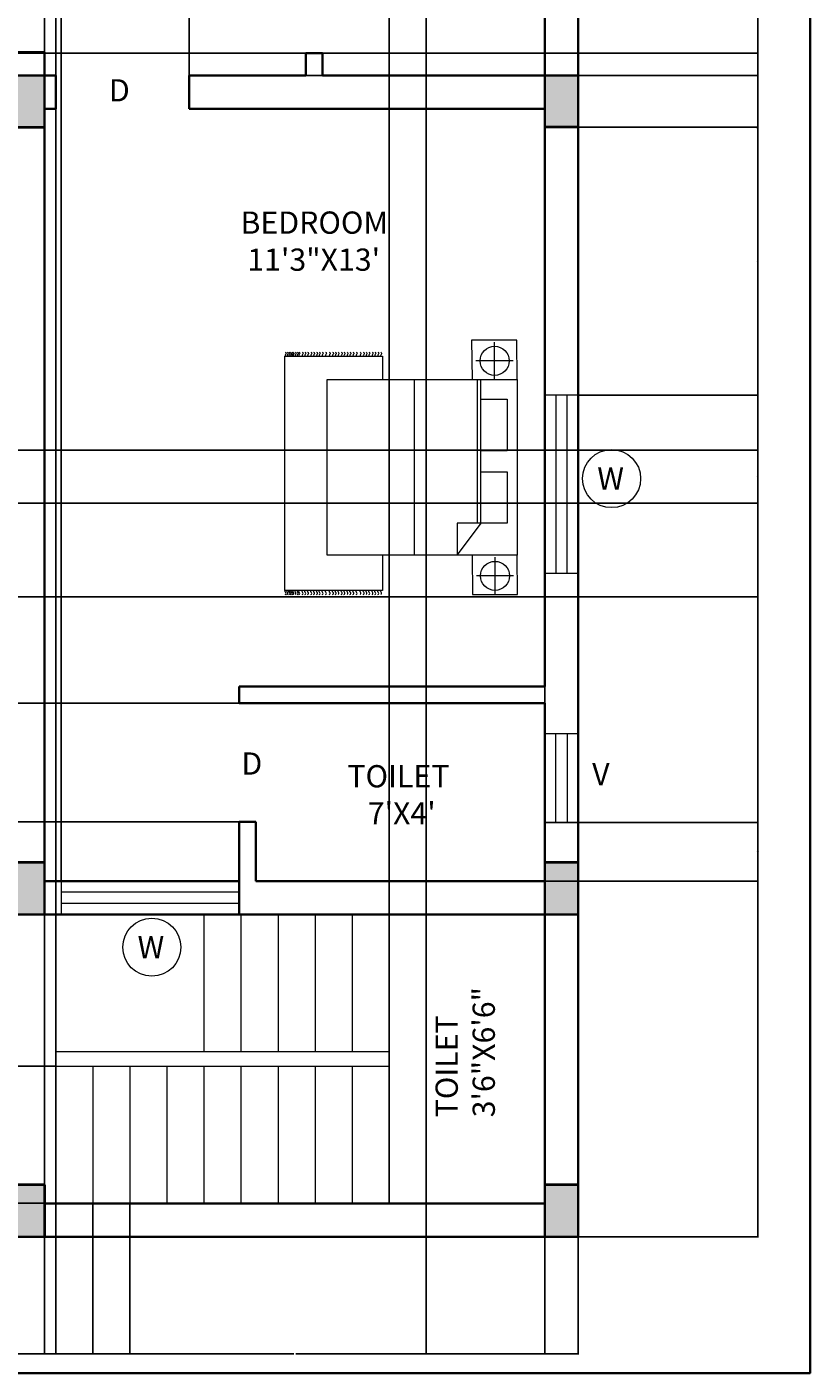
# Model space of a CAD drawing. Units: inches. Extents: x 2243 to 2668, y 14541 to 15226.
# Tile 2 of 5: x 2456 to 2668, y 14541 to 14904. Entities that reach past the tile are written whole.
import ezdxf

# ---------------------------------------------------------------- set-up
doc = ezdxf.new("R2010")
doc.units = ezdxf.units.IN
doc.header["$MEASUREMENT"] = 0
for name, color, linetype, lineweight in [('A-ANNO-DIMS', 2, 'Continuous', 18), ('A-ANNO-SYMB', 3, 'Continuous', 18), ('A-ANNO-TTLB', 7, 'Continuous', 35), ('A-AREA-IDEN', 7, 'Continuous', 18), ('A-COLS', 7, 'Continuous', 40), ('A-COLS-PATT', 7, 'Continuous', 13), ('A-FLOR-STRS', 7, 'Continuous', 18), ('A-FURN', 8, 'Continuous', 18), ('A-GLAZ', 4, 'Continuous', 18), ('A-GLAZ-VENT', 4, 'Continuous', 18), ('A-WALL', 7, 'Continuous', 35)]:
    doc.layers.add(name, color=color, linetype=linetype, lineweight=lineweight)
doc.styles.get("Standard").update_dxf_attribs({"font": 'arial.ttf'})
doc.dimstyles.get("Standard").update_dxf_attribs({"dimtxt": 0.18, "dimasz": 0.18, "dimexe": 0.18, "dimexo": 0.0625, "dimgap": 0.09, "dimtad": 0, "dimtih": 1, "dimtoh": 1, "dimdec": 4, "dimzin": 0, "dimdsep": 46, "dimtxsty": 'Standard', "dimcen": 0.09, "dimadec": 0, "dimazin": 0, "dimtfac": 1, "dimtdec": 4, "dimtofl": 0, "dimtmove": 0, "dimatfit": 3, "dimfxl": 1, "dimtolj": 1, "dimtzin": 0, "dimarcsym": 0})

# ---------------------------------------------------------------- blocks, each defined once
blk = doc.blocks.new('BED-DOUBLE-WITH-NIGHTSTANDS')
for p, q in [((56.59, 58.08), (56.59, 68.14)), ((0, 64.36), (26.37, 64.36)), ((0, 1.12), (0, 64.36)), ((26.37, 64.36), (26.37, 58.06)), ((61.62, 63.11), (51.56, 63.11)), ((34.96, 10.66), (34.96, 58.08)), ((52, 19.27), (52, 58.08)), ((52.82, 19.32), (52.82, 58.08)), ((52.82, 19.32), (46.47, 10.71)), ((52.82, 19.27), (46.47, 19.27)), ((46.47, 19.27), (46.47, 10.71)), ((26.37, 10.66), (26.37, 1.12)), ((56.69, 0.03), (56.69, 10.09)), ((61.72, 5.06), (51.66, 5.06)), ((26.37, 1.12), (0, 1.12))]:
    blk.add_line(p, q)
for points in [[(50.39, 68.71), (50.5, 58.08), (62.68, 58.08), (62.58, 68.71)], [(62.68, 10.66), (11.36, 10.66), (11.36, 58.08), (62.68, 58.08)], [(59.98, 38.83), (52.82, 38.83), (52.82, 52.73), (59.98, 52.73)], [(59.98, 19.27), (52.82, 19.27), (52.82, 33.16), (59.98, 33.16)], [(50.5, 10.66), (50.6, 0.03), (62.78, 0.03), (62.68, 10.66)]]:
    blk.add_lwpolyline(points, close=True)
for centre in [(56.59, 63.11), (56.69, 5.06)]:
    blk.add_circle(centre, 3.92)
for points, knots in [([(0.07, 65.48), (0.19, 65.39), (0.43, 65.19), (0.19, 64.85), (0.02, 64.57), (0.13, 64.42), (0.18, 64.36)], [0, 0, 0, 0, 0.400747, 0.791423, 1.067667, 1.29709, 1.29709, 1.29709, 1.29709]), ([(0.57, 65.48), (0.7, 65.39), (0.94, 65.19), (0.7, 64.85), (0.52, 64.57), (0.63, 64.42), (0.68, 64.36)], [0, 0, 0, 0, 0.400747, 0.791423, 1.067667, 1.29709, 1.29709, 1.29709, 1.29709]), ([(1.06, 65.48), (1.18, 65.39), (1.42, 65.19), (1.18, 64.85), (1.01, 64.57), (1.11, 64.42), (1.16, 64.36)], [0, 0, 0, 0, 0.400747, 0.791423, 1.067667, 1.29709, 1.29709, 1.29709, 1.29709]), ([(1.46, 65.48), (1.58, 65.39), (1.82, 65.19), (1.58, 64.85), (1.4, 64.57), (1.51, 64.42), (1.56, 64.36)], [0, 0, 0, 0, 0.400747, 0.791423, 1.067667, 1.29709, 1.29709, 1.29709, 1.29709]), ([(1.88, 65.48), (2, 65.39), (2.24, 65.19), (2, 64.85), (1.82, 64.57), (1.93, 64.42), (1.98, 64.36)], [0, 0, 0, 0, 0.400747, 0.791423, 1.067667, 1.29709, 1.29709, 1.29709, 1.29709]), ([(2.18, 65.48), (2.31, 65.39), (2.55, 65.19), (2.31, 64.85), (2.13, 64.57), (2.24, 64.42), (2.29, 64.36)], [0, 0, 0, 0, 0.400747, 0.791423, 1.067667, 1.29709, 1.29709, 1.29709, 1.29709]), ([(2.76, 65.48), (2.88, 65.39), (3.12, 65.19), (2.88, 64.85), (2.71, 64.57), (2.81, 64.42), (2.86, 64.36)], [0, 0, 0, 0, 0.400747, 0.791423, 1.067667, 1.29709, 1.29709, 1.29709, 1.29709]), ([(3.32, 65.48), (3.45, 65.39), (3.7, 65.2), (3.44, 64.85), (3.27, 64.57), (3.38, 64.42), (3.43, 64.36)], [0, 0, 0, 0, 0.407265, 0.802015, 1.07826, 1.307683, 1.307683, 1.307683, 1.307683]), ([(3.75, 65.48), (3.88, 65.39), (4.11, 65.19), (3.88, 64.85), (3.7, 64.57), (3.81, 64.42), (3.86, 64.36)], [0, 0, 0, 0, 0.400747, 0.791423, 1.067667, 1.29709, 1.29709, 1.29709, 1.29709]), ([(4.64, 65.48), (4.76, 65.39), (5, 65.19), (4.76, 64.85), (4.58, 64.57), (4.69, 64.42), (4.74, 64.36)], [0, 0, 0, 0, 0.400747, 0.791423, 1.067667, 1.29709, 1.29709, 1.29709, 1.29709]), ([(5.36, 65.48), (5.49, 65.39), (5.73, 65.19), (5.49, 64.85), (5.31, 64.57), (5.42, 64.42), (5.47, 64.36)], [0, 0, 0, 0, 0.400747, 0.791423, 1.067667, 1.29709, 1.29709, 1.29709, 1.29709]), ([(6.12, 65.48), (6.24, 65.39), (6.48, 65.19), (6.24, 64.85), (6.07, 64.57), (6.17, 64.42), (6.22, 64.36)], [0, 0, 0, 0, 0.400747, 0.791423, 1.067667, 1.29709, 1.29709, 1.29709, 1.29709]), ([(7, 65.48), (7.12, 65.39), (7.36, 65.19), (7.12, 64.85), (6.95, 64.57), (7.05, 64.42), (7.1, 64.36)], [0, 0, 0, 0, 0.400747, 0.791423, 1.067667, 1.29709, 1.29709, 1.29709, 1.29709]), ([(7.73, 65.48), (7.85, 65.39), (8.09, 65.19), (7.85, 64.85), (7.68, 64.57), (7.78, 64.42), (7.83, 64.36)], [0, 0, 0, 0, 0.400747, 0.791423, 1.067667, 1.29709, 1.29709, 1.29709, 1.29709]), ([(8.54, 65.48), (8.66, 65.39), (8.9, 65.19), (8.66, 64.85), (8.49, 64.57), (8.6, 64.42), (8.65, 64.36)], [0, 0, 0, 0, 0.400747, 0.791423, 1.067667, 1.29709, 1.29709, 1.29709, 1.29709]), ([(9.23, 65.48), (9.35, 65.39), (9.59, 65.19), (9.35, 64.85), (9.18, 64.57), (9.29, 64.42), (9.34, 64.36)], [0, 0, 0, 0, 0.400747, 0.791423, 1.067667, 1.29709, 1.29709, 1.29709, 1.29709]), ([(10.05, 65.48), (10.17, 65.39), (10.41, 65.19), (10.17, 64.85), (10, 64.57), (10.1, 64.42), (10.15, 64.36)], [0, 0, 0, 0, 0.400747, 0.791423, 1.067667, 1.29709, 1.29709, 1.29709, 1.29709]), ([(10.93, 65.48), (11.05, 65.39), (11.29, 65.19), (11.05, 64.85), (10.88, 64.57), (10.99, 64.42), (11.03, 64.36)], [0, 0, 0, 0, 0.400747, 0.791423, 1.067667, 1.29709, 1.29709, 1.29709, 1.29709]), ([(11.97, 65.48), (12.09, 65.39), (12.33, 65.19), (12.09, 64.85), (11.92, 64.57), (12.02, 64.42), (12.07, 64.36)], [0, 0, 0, 0, 0.400747, 0.791423, 1.067667, 1.29709, 1.29709, 1.29709, 1.29709]), ([(12.85, 65.48), (12.97, 65.39), (13.21, 65.19), (12.97, 64.85), (12.8, 64.57), (12.9, 64.42), (12.95, 64.36)], [0, 0, 0, 0, 0.400747, 0.791423, 1.067667, 1.29709, 1.29709, 1.29709, 1.29709]), ([(13.58, 65.48), (13.7, 65.39), (13.94, 65.19), (13.7, 64.85), (13.53, 64.57), (13.63, 64.42), (13.68, 64.36)], [0, 0, 0, 0, 0.400747, 0.791423, 1.067667, 1.29709, 1.29709, 1.29709, 1.29709]), ([(14.33, 65.48), (14.45, 65.39), (14.69, 65.19), (14.45, 64.85), (14.28, 64.57), (14.38, 64.42), (14.43, 64.36)], [0, 0, 0, 0, 0.400747, 0.791423, 1.067667, 1.29709, 1.29709, 1.29709, 1.29709]), ([(15.21, 65.48), (15.33, 65.39), (15.57, 65.19), (15.33, 64.85), (15.16, 64.57), (15.27, 64.42), (15.32, 64.36)], [0, 0, 0, 0, 0.400747, 0.791423, 1.067667, 1.29709, 1.29709, 1.29709, 1.29709]), ([(15.94, 65.48), (16.06, 65.39), (16.3, 65.19), (16.06, 64.85), (15.89, 64.57), (15.99, 64.42), (16.04, 64.36)], [0, 0, 0, 0, 0.400747, 0.791423, 1.067667, 1.29709, 1.29709, 1.29709, 1.29709]), ([(16.76, 65.48), (16.88, 65.39), (17.12, 65.19), (16.88, 64.85), (16.7, 64.57), (16.81, 64.42), (16.86, 64.36)], [0, 0, 0, 0, 0.400747, 0.791423, 1.067667, 1.29709, 1.29709, 1.29709, 1.29709]), ([(17.53, 65.48), (17.65, 65.39), (17.89, 65.19), (17.65, 64.85), (17.48, 64.57), (17.59, 64.42), (17.64, 64.36)], [0, 0, 0, 0, 0.400747, 0.791423, 1.067667, 1.29709, 1.29709, 1.29709, 1.29709]), ([(18.35, 65.48), (18.47, 65.39), (18.71, 65.19), (18.47, 64.85), (18.3, 64.57), (18.4, 64.42), (18.45, 64.36)], [0, 0, 0, 0, 0.400747, 0.791423, 1.067667, 1.29709, 1.29709, 1.29709, 1.29709]), ([(19.23, 65.48), (19.35, 65.39), (19.59, 65.19), (19.35, 64.85), (19.18, 64.57), (19.29, 64.42), (19.33, 64.36)], [0, 0, 0, 0, 0.400747, 0.791423, 1.067667, 1.29709, 1.29709, 1.29709, 1.29709]), ([(20.27, 65.48), (20.39, 65.39), (20.63, 65.19), (20.39, 64.85), (20.22, 64.57), (20.32, 64.42), (20.37, 64.36)], [0, 0, 0, 0, 0.400747, 0.791423, 1.067667, 1.29709, 1.29709, 1.29709, 1.29709]), ([(21.15, 65.48), (21.27, 65.39), (21.51, 65.19), (21.27, 64.85), (21.1, 64.57), (21.21, 64.42), (21.25, 64.36)], [0, 0, 0, 0, 0.400747, 0.791423, 1.067667, 1.29709, 1.29709, 1.29709, 1.29709]), ([(21.88, 65.48), (22, 65.39), (22.24, 65.19), (22, 64.85), (21.83, 64.57), (21.93, 64.42), (21.98, 64.36)], [0, 0, 0, 0, 0.400747, 0.791423, 1.067667, 1.29709, 1.29709, 1.29709, 1.29709]), ([(22.63, 65.48), (22.75, 65.39), (22.99, 65.19), (22.75, 64.85), (22.58, 64.57), (22.69, 64.42), (22.73, 64.36)], [0, 0, 0, 0, 0.400747, 0.791423, 1.067667, 1.29709, 1.29709, 1.29709, 1.29709]), ([(23.51, 65.48), (23.63, 65.39), (23.87, 65.19), (23.63, 64.85), (23.46, 64.57), (23.57, 64.42), (23.62, 64.36)], [0, 0, 0, 0, 0.400747, 0.791423, 1.067667, 1.29709, 1.29709, 1.29709, 1.29709]), ([(24.24, 65.48), (24.36, 65.39), (24.6, 65.19), (24.36, 64.85), (24.19, 64.57), (24.3, 64.42), (24.34, 64.36)], [0, 0, 0, 0, 0.400747, 0.791423, 1.067667, 1.29709, 1.29709, 1.29709, 1.29709]), ([(25.06, 65.48), (25.18, 65.39), (25.42, 65.19), (25.18, 64.85), (25.01, 64.57), (25.11, 64.42), (25.16, 64.36)], [0, 0, 0, 0, 0.400747, 0.791423, 1.067667, 1.29709, 1.29709, 1.29709, 1.29709]), ([(25.84, 65.48), (25.96, 65.39), (26.2, 65.19), (25.96, 64.85), (25.78, 64.57), (25.89, 64.42), (25.94, 64.36)], [0, 0, 0, 0, 0.400747, 0.791423, 1.067667, 1.29709, 1.29709, 1.29709, 1.29709]), ([(0.07, 0), (0.19, 0.1), (0.43, 0.29), (0.19, 0.63), (0.02, 0.91), (0.13, 1.06), (0.18, 1.13)], [0, 0, 0, 0, 0.400747, 0.791423, 1.067667, 1.29709, 1.29709, 1.29709, 1.29709]), ([(0.55, 0), (0.67, 0.1), (0.91, 0.29), (0.67, 0.63), (0.49, 0.91), (0.6, 1.06), (0.65, 1.13)], [0, 0, 0, 0, 0.400747, 0.791423, 1.067667, 1.29709, 1.29709, 1.29709, 1.29709]), ([(1.03, 0), (1.15, 0.1), (1.39, 0.29), (1.15, 0.63), (0.98, 0.91), (1.09, 1.06), (1.13, 1.13)], [0, 0, 0, 0, 0.400747, 0.791423, 1.067667, 1.29709, 1.29709, 1.29709, 1.29709]), ([(1.43, 0), (1.55, 0.1), (1.79, 0.29), (1.55, 0.63), (1.38, 0.91), (1.48, 1.06), (1.53, 1.13)], [0, 0, 0, 0, 0.400747, 0.791423, 1.067667, 1.29709, 1.29709, 1.29709, 1.29709]), ([(1.85, 0), (1.97, 0.1), (2.21, 0.29), (1.97, 0.63), (1.8, 0.91), (1.9, 1.05), (1.94, 1.12)], [0, 0, 0, 0, 0.400747, 0.791423, 1.067667, 1.283686, 1.283686, 1.283686, 1.283686]), ([(2.16, 0), (2.28, 0.1), (2.52, 0.29), (2.28, 0.63), (2.11, 0.91), (2.21, 1.05), (2.25, 1.12)], [0, 0, 0, 0, 0.400747, 0.791423, 1.067667, 1.283686, 1.283686, 1.283686, 1.283686]), ([(2.73, 0), (2.85, 0.1), (3.09, 0.29), (2.85, 0.63), (2.68, 0.91), (2.78, 1.05), (2.82, 1.12)], [0, 0, 0, 0, 0.400747, 0.791423, 1.067667, 1.283686, 1.283686, 1.283686, 1.283686]), ([(3.32, 0), (3.45, 0.1), (3.69, 0.29), (3.45, 0.63), (3.27, 0.91), (3.38, 1.05), (3.42, 1.12)], [0, 0, 0, 0, 0.402903, 0.794912, 1.071156, 1.287177, 1.287177, 1.287177, 1.287177]), ([(3.75, 0), (3.88, 0.1), (4.11, 0.29), (3.88, 0.63), (3.7, 0.91), (3.8, 1.05), (3.85, 1.12)], [0, 0, 0, 0, 0.400747, 0.791423, 1.067667, 1.283686, 1.283686, 1.283686, 1.283686]), ([(4.64, 0), (4.76, 0.1), (5, 0.29), (4.76, 0.63), (4.59, 0.91), (4.69, 1.05), (4.73, 1.12)], [0, 0, 0, 0, 0.400747, 0.791423, 1.067667, 1.283686, 1.283686, 1.283686, 1.283686]), ([(5.36, 0), (5.49, 0.1), (5.73, 0.29), (5.49, 0.63), (5.31, 0.91), (5.42, 1.06), (5.47, 1.13)], [0, 0, 0, 0, 0.400747, 0.791423, 1.067667, 1.29709, 1.29709, 1.29709, 1.29709]), ([(6.12, 0), (6.24, 0.1), (6.48, 0.29), (6.24, 0.63), (6.07, 0.91), (6.17, 1.06), (6.22, 1.13)], [0, 0, 0, 0, 0.400747, 0.791423, 1.067667, 1.29709, 1.29709, 1.29709, 1.29709]), ([(7, 0), (7.12, 0.1), (7.36, 0.29), (7.12, 0.63), (6.95, 0.91), (7.05, 1.06), (7.1, 1.13)], [0, 0, 0, 0, 0.400747, 0.791423, 1.067667, 1.29709, 1.29709, 1.29709, 1.29709]), ([(7.73, 0), (7.85, 0.1), (8.09, 0.29), (7.85, 0.63), (7.68, 0.91), (7.78, 1.06), (7.83, 1.13)], [0, 0, 0, 0, 0.400747, 0.791423, 1.067667, 1.29709, 1.29709, 1.29709, 1.29709]), ([(8.54, 0), (8.66, 0.1), (8.9, 0.29), (8.66, 0.63), (8.49, 0.91), (8.6, 1.06), (8.65, 1.13)], [0, 0, 0, 0, 0.400747, 0.791423, 1.067667, 1.29709, 1.29709, 1.29709, 1.29709]), ([(9.23, 0), (9.35, 0.1), (9.59, 0.29), (9.35, 0.63), (9.18, 0.91), (9.29, 1.06), (9.34, 1.13)], [0, 0, 0, 0, 0.400747, 0.791423, 1.067667, 1.29709, 1.29709, 1.29709, 1.29709]), ([(10.05, 0), (10.17, 0.1), (10.41, 0.29), (10.17, 0.63), (10, 0.91), (10.1, 1.06), (10.15, 1.13)], [0, 0, 0, 0, 0.400747, 0.791423, 1.067667, 1.29709, 1.29709, 1.29709, 1.29709]), ([(10.93, 0), (11.05, 0.1), (11.29, 0.29), (11.05, 0.63), (10.88, 0.91), (10.99, 1.06), (11.03, 1.13)], [0, 0, 0, 0, 0.400747, 0.791423, 1.067667, 1.29709, 1.29709, 1.29709, 1.29709]), ([(11.97, 0), (12.09, 0.1), (12.33, 0.29), (12.09, 0.63), (11.92, 0.91), (12.02, 1.06), (12.07, 1.13)], [0, 0, 0, 0, 0.400747, 0.791423, 1.067667, 1.29709, 1.29709, 1.29709, 1.29709]), ([(12.85, 0), (12.97, 0.1), (13.21, 0.29), (12.97, 0.63), (12.8, 0.91), (12.9, 1.06), (12.95, 1.13)], [0, 0, 0, 0, 0.400747, 0.791423, 1.067667, 1.29709, 1.29709, 1.29709, 1.29709]), ([(13.58, 0), (13.7, 0.1), (13.94, 0.29), (13.7, 0.63), (13.53, 0.91), (13.63, 1.06), (13.68, 1.13)], [0, 0, 0, 0, 0.400747, 0.791423, 1.067667, 1.29709, 1.29709, 1.29709, 1.29709]), ([(14.33, 0), (14.45, 0.1), (14.69, 0.29), (14.45, 0.63), (14.28, 0.91), (14.38, 1.06), (14.43, 1.13)], [0, 0, 0, 0, 0.400747, 0.791423, 1.067667, 1.29709, 1.29709, 1.29709, 1.29709]), ([(15.21, 0), (15.33, 0.1), (15.57, 0.29), (15.33, 0.63), (15.16, 0.91), (15.27, 1.06), (15.32, 1.13)], [0, 0, 0, 0, 0.400747, 0.791423, 1.067667, 1.29709, 1.29709, 1.29709, 1.29709]), ([(15.94, 0), (16.06, 0.1), (16.3, 0.29), (16.06, 0.63), (15.89, 0.91), (15.99, 1.06), (16.04, 1.13)], [0, 0, 0, 0, 0.400747, 0.791423, 1.067667, 1.29709, 1.29709, 1.29709, 1.29709]), ([(16.76, 0), (16.88, 0.1), (17.12, 0.29), (16.88, 0.63), (16.7, 0.91), (16.81, 1.06), (16.86, 1.13)], [0, 0, 0, 0, 0.400747, 0.791423, 1.067667, 1.29709, 1.29709, 1.29709, 1.29709]), ([(17.53, 0), (17.65, 0.1), (17.89, 0.29), (17.65, 0.63), (17.48, 0.91), (17.59, 1.06), (17.64, 1.13)], [0, 0, 0, 0, 0.400747, 0.791423, 1.067667, 1.29709, 1.29709, 1.29709, 1.29709]), ([(18.35, 0), (18.47, 0.1), (18.71, 0.29), (18.47, 0.63), (18.3, 0.91), (18.4, 1.06), (18.45, 1.13)], [0, 0, 0, 0, 0.400747, 0.791423, 1.067667, 1.29709, 1.29709, 1.29709, 1.29709]), ([(19.23, 0), (19.35, 0.1), (19.59, 0.29), (19.35, 0.63), (19.18, 0.91), (19.29, 1.06), (19.33, 1.13)], [0, 0, 0, 0, 0.400747, 0.791423, 1.067667, 1.29709, 1.29709, 1.29709, 1.29709]), ([(20.27, 0), (20.39, 0.1), (20.63, 0.29), (20.39, 0.63), (20.22, 0.91), (20.32, 1.06), (20.37, 1.13)], [0, 0, 0, 0, 0.400747, 0.791423, 1.067667, 1.29709, 1.29709, 1.29709, 1.29709]), ([(21.15, 0), (21.27, 0.1), (21.51, 0.29), (21.27, 0.63), (21.1, 0.91), (21.21, 1.06), (21.25, 1.13)], [0, 0, 0, 0, 0.400747, 0.791423, 1.067667, 1.29709, 1.29709, 1.29709, 1.29709]), ([(21.88, 0), (22, 0.1), (22.24, 0.29), (22, 0.63), (21.83, 0.91), (21.93, 1.06), (21.98, 1.13)], [0, 0, 0, 0, 0.400747, 0.791423, 1.067667, 1.29709, 1.29709, 1.29709, 1.29709]), ([(22.63, 0), (22.75, 0.1), (22.99, 0.29), (22.75, 0.63), (22.58, 0.91), (22.69, 1.06), (22.73, 1.13)], [0, 0, 0, 0, 0.400747, 0.791423, 1.067667, 1.29709, 1.29709, 1.29709, 1.29709]), ([(23.51, 0), (23.63, 0.1), (23.87, 0.29), (23.63, 0.63), (23.46, 0.91), (23.57, 1.06), (23.62, 1.13)], [0, 0, 0, 0, 0.400747, 0.791423, 1.067667, 1.29709, 1.29709, 1.29709, 1.29709]), ([(24.24, 0), (24.36, 0.1), (24.6, 0.29), (24.36, 0.63), (24.19, 0.91), (24.3, 1.06), (24.34, 1.13)], [0, 0, 0, 0, 0.400747, 0.791423, 1.067667, 1.29709, 1.29709, 1.29709, 1.29709]), ([(25.06, 0), (25.18, 0.1), (25.42, 0.29), (25.18, 0.63), (25.01, 0.91), (25.11, 1.06), (25.16, 1.13)], [0, 0, 0, 0, 0.400747, 0.791423, 1.067667, 1.29709, 1.29709, 1.29709, 1.29709]), ([(25.84, 0), (25.96, 0.1), (26.2, 0.29), (25.96, 0.63), (25.78, 0.91), (25.89, 1.06), (25.94, 1.13)], [0, 0, 0, 0, 0.400747, 0.791423, 1.067667, 1.29709, 1.29709, 1.29709, 1.29709])]:
    blk.add_open_spline(points, degree=3, knots=knots)
blk = doc.blocks.new('WIN-48IN')
for p, q in [((0, 9), (0, 0)), ((48, 9), (0, 9)), ((48, 0), (48, 9)), ((48, 6), (0, 6)), ((0, 3), (48, 3)), ((0, 0), (48, 0))]:
    blk.add_line(p, q)
blk = doc.blocks.new('TAG-WINDOW-W')
blk.add_circle((7.84, 7.84), 7.84)
at = {"insert": (3.99, 10.84), "char_height": 6, "attachment_point": 1}
blk.add_mtext_dynamic_manual_height_columns('W', width=14.3449, gutter_width=30, heights=[0], dxfattribs=at)
blk = doc.blocks.new('VENT-24IN')
for p, q in [((0, 24), (9, 24)), ((0, 0), (0, 24)), ((3, 0), (3, 24)), ((6, 24), (6, 0)), ((9, 24), (9, 0)), ((9, 0), (0, 0))]:
    blk.add_line(p, q)
blk = doc.blocks.new('*D18')
at = {"layer": 'A-ANNO-DIMS', "color": 0, "lineweight": -2, "transparency": 16777216}
for p, q in [((2605.02, 15176.14), (2653.58, 15176.14)), ((2653.4, 15175.96), (2653.4, 14877.07)), ((2653.4, 14577.82), (2653.4, 14876.7)), ((2605.02, 14577.64), (2653.58, 14577.64))]:
    blk.add_line(p, q, dxfattribs=at)
at = {"layer": 'A-ANNO-DIMS', "color": 0, "transparency": 16777216}
for points in [[(2653.37, 15175.96), (2653.43, 15175.96), (2653.4, 15176.14)], [(2653.37, 14577.82), (2653.43, 14577.82), (2653.4, 14577.64)]]:
    blk.add_solid(points, dxfattribs=at)
at = {"layer": 'Defpoints', "color": 0, "transparency": 16777216}
for p in [(2604.96, 15176.14), (2653.4, 15176.14), (2604.96, 14577.64)]:
    blk.add_point(p, dxfattribs=at)
at = {"layer": 'A-ANNO-DIMS', "color": 0, "transparency": 16777216, "insert": (2653.4, 14876.89), "char_height": 0.18, "attachment_point": 5}
blk.add_mtext('\\A1;598.5', dxfattribs=at)
blk = doc.blocks.new('*D20')
at = {"layer": 'A-ANNO-DIMS', "color": 0, "lineweight": -2, "transparency": 16777216}
for p, q in [((2451.96, 14577.57), (2451.96, 14545.86)), ((2604.96, 14577.57), (2604.96, 14545.86)), ((2452.14, 14546.04), (2528.18, 14546.04)), ((2604.78, 14546.04), (2528.74, 14546.04))]:
    blk.add_line(p, q, dxfattribs=at)
at = {"layer": 'A-ANNO-DIMS', "color": 0, "transparency": 16777216}
for points in [[(2452.14, 14546.07), (2452.14, 14546.01), (2451.96, 14546.04)], [(2604.78, 14546.07), (2604.78, 14546.01), (2604.96, 14546.04)]]:
    blk.add_solid(points, dxfattribs=at)
at = {"layer": 'Defpoints', "color": 0, "transparency": 16777216}
for p in [(2451.96, 14577.64), (2604.96, 14577.64), (2604.96, 14546.04)]:
    blk.add_point(p, dxfattribs=at)
at = {"layer": 'A-ANNO-DIMS', "color": 0, "transparency": 16777216, "insert": (2528.46, 14546.04), "char_height": 0.18, "attachment_point": 5}
blk.add_mtext('\\A1;153', dxfattribs=at)
blk = doc.blocks.new('*D29')
at = {"layer": 'A-ANNO-DIMS', "color": 0, "lineweight": -2, "transparency": 16777216}
for p, q in [((2596.02, 14689.49), (2653.58, 14689.49)), ((2653.4, 14689.31), (2653.4, 14681.75)), ((2653.4, 14673.82), (2653.4, 14681.38)), ((2596.02, 14673.64), (2653.58, 14673.64))]:
    blk.add_line(p, q, dxfattribs=at)
at = {"layer": 'A-ANNO-DIMS', "color": 0, "transparency": 16777216}
for points in [[(2653.37, 14689.31), (2653.43, 14689.31), (2653.4, 14689.49)], [(2653.37, 14673.82), (2653.43, 14673.82), (2653.4, 14673.64)]]:
    blk.add_solid(points, dxfattribs=at)
at = {"layer": 'Defpoints', "color": 0, "transparency": 16777216}
for p in [(2595.96, 14689.49), (2653.4, 14689.49), (2595.96, 14673.64)]:
    blk.add_point(p, dxfattribs=at)
at = {"layer": 'A-ANNO-DIMS', "color": 0, "transparency": 16777216, "insert": (2653.4, 14681.56), "char_height": 0.18, "attachment_point": 5}
blk.add_mtext('\\A1;15.854', dxfattribs=at)
blk = doc.blocks.new('*D30')
at = {"layer": 'A-ANNO-DIMS', "color": 0, "lineweight": -2, "transparency": 16777216}
for p, q in [((2605.02, 14877.14), (2653.58, 14877.14)), ((2653.4, 14876.96), (2653.4, 14841.15)), ((2653.4, 14804.98), (2653.4, 14840.79)), ((2605.02, 14804.8), (2653.58, 14804.8))]:
    blk.add_line(p, q, dxfattribs=at)
at = {"layer": 'A-ANNO-DIMS', "color": 0, "transparency": 16777216}
for points in [[(2653.37, 14876.96), (2653.43, 14876.96), (2653.4, 14877.14)], [(2653.37, 14804.98), (2653.43, 14804.98), (2653.4, 14804.8)]]:
    blk.add_solid(points, dxfattribs=at)
at = {"layer": 'Defpoints', "color": 0, "transparency": 16777216}
for p in [(2604.96, 14877.14), (2653.4, 14877.14), (2604.96, 14804.8)]:
    blk.add_point(p, dxfattribs=at)
at = {"layer": 'A-ANNO-DIMS', "color": 0, "transparency": 16777216, "insert": (2653.4, 14840.97), "char_height": 0.18, "attachment_point": 5}
blk.add_mtext('\\A1;72.34', dxfattribs=at)
blk = doc.blocks.new('*D36')
at = {"layer": 'A-ANNO-DIMS', "color": 0, "lineweight": -2, "transparency": 16777216}
for p, q in [((2460.96, 14673.7), (2460.96, 15225.04)), ((2461.14, 15224.86), (2462.95, 15224.86)), ((2465.28, 15224.86), (2463.47, 15224.86)), ((2465.46, 14673.7), (2465.46, 15225.04))]:
    blk.add_line(p, q, dxfattribs=at)
at = {"layer": 'A-ANNO-DIMS', "color": 0, "transparency": 16777216}
for points in [[(2461.14, 15224.89), (2461.14, 15224.83), (2460.96, 15224.86)], [(2465.28, 15224.89), (2465.28, 15224.83), (2465.46, 15224.86)]]:
    blk.add_solid(points, dxfattribs=at)
at = {"layer": 'Defpoints', "color": 0, "transparency": 16777216}
for p in [(2465.46, 15224.86), (2460.96, 14673.64), (2465.46, 14673.64)]:
    blk.add_point(p, dxfattribs=at)
at = {"layer": 'A-ANNO-DIMS', "color": 0, "transparency": 16777216, "insert": (2463.21, 15224.86), "char_height": 0.18, "attachment_point": 5}
blk.add_mtext('\\A1;4.5', dxfattribs=at)
blk = doc.blocks.new('*D37')
at = {"layer": 'A-ANNO-DIMS', "color": 0, "lineweight": -2, "transparency": 16777216}
for p, q in [((2463.96, 14586.7), (2463.96, 15225.04)), ((2464.14, 15224.86), (2508.74, 15224.86)), ((2553.78, 15224.86), (2509.18, 15224.86)), ((2553.96, 14586.7), (2553.96, 15225.04))]:
    blk.add_line(p, q, dxfattribs=at)
at = {"layer": 'A-ANNO-DIMS', "color": 0, "transparency": 16777216}
for points in [[(2464.14, 15224.89), (2464.14, 15224.83), (2463.96, 15224.86)], [(2553.78, 15224.89), (2553.78, 15224.83), (2553.96, 15224.86)]]:
    blk.add_solid(points, dxfattribs=at)
at = {"layer": 'Defpoints', "color": 0, "transparency": 16777216}
for p in [(2553.96, 15224.86), (2463.96, 14586.64), (2553.96, 14586.64)]:
    blk.add_point(p, dxfattribs=at)
at = {"layer": 'A-ANNO-DIMS', "color": 0, "transparency": 16777216, "insert": (2508.96, 15224.86), "char_height": 0.18, "attachment_point": 5}
blk.add_mtext('\\A1;90', dxfattribs=at)
blk = doc.blocks.new('*D38')
at = {"layer": 'A-ANNO-DIMS', "color": 0, "lineweight": -2, "transparency": 16777216}
for p, q in [((2463.9, 14623.64), (2243.57, 14623.64)), ((2243.75, 14623.46), (2243.75, 14605.32)), ((2243.75, 14586.82), (2243.75, 14604.95)), ((2463.9, 14586.64), (2243.57, 14586.64))]:
    blk.add_line(p, q, dxfattribs=at)
at = {"layer": 'A-ANNO-DIMS', "color": 0, "transparency": 16777216}
for points in [[(2243.72, 14623.46), (2243.78, 14623.46), (2243.75, 14623.64)], [(2243.72, 14586.82), (2243.78, 14586.82), (2243.75, 14586.64)]]:
    blk.add_solid(points, dxfattribs=at)
at = {"layer": 'Defpoints', "color": 0, "transparency": 16777216}
for p in [(2243.75, 14623.64), (2463.96, 14623.64), (2463.96, 14586.64)]:
    blk.add_point(p, dxfattribs=at)
at = {"layer": 'A-ANNO-DIMS', "color": 0, "transparency": 16777216, "insert": (2243.75, 14605.14), "char_height": 0.18, "attachment_point": 5}
blk.add_mtext('\\A1;37', dxfattribs=at)
blk = doc.blocks.new('*D39')
at = {"layer": 'A-ANNO-DIMS', "color": 0, "lineweight": -2, "transparency": 16777216}
for p, q in [((2473.96, 14586.57), (2473.96, 14545.86)), ((2483.96, 14586.57), (2483.96, 14545.86)), ((2474.14, 14546.04), (2478.75, 14546.04)), ((2483.78, 14546.04), (2479.17, 14546.04))]:
    blk.add_line(p, q, dxfattribs=at)
at = {"layer": 'A-ANNO-DIMS', "color": 0, "transparency": 16777216}
for points in [[(2474.14, 14546.07), (2474.14, 14546.01), (2473.96, 14546.04)], [(2483.78, 14546.07), (2483.78, 14546.01), (2483.96, 14546.04)]]:
    blk.add_solid(points, dxfattribs=at)
at = {"layer": 'Defpoints', "color": 0, "transparency": 16777216}
for p in [(2473.96, 14586.64), (2483.96, 14586.64), (2483.96, 14546.04)]:
    blk.add_point(p, dxfattribs=at)
at = {"layer": 'A-ANNO-DIMS', "color": 0, "transparency": 16777216, "insert": (2478.96, 14546.04), "char_height": 0.18, "attachment_point": 5}
blk.add_mtext('\\A1;10', dxfattribs=at)
blk = doc.blocks.new('*D48')
at = {"layer": 'A-ANNO-DIMS', "color": 0, "lineweight": -2, "transparency": 16777216}
for p, q in [((2463.96, 14891.2), (2463.96, 15225.04)), ((2464.14, 15224.86), (2481.74, 15224.86)), ((2499.78, 15224.86), (2482.18, 15224.86)), ((2499.96, 14891.2), (2499.96, 15225.04))]:
    blk.add_line(p, q, dxfattribs=at)
at = {"layer": 'A-ANNO-DIMS', "color": 0, "transparency": 16777216}
for points in [[(2464.14, 15224.89), (2464.14, 15224.83), (2463.96, 15224.86)], [(2499.78, 15224.89), (2499.78, 15224.83), (2499.96, 15224.86)]]:
    blk.add_solid(points, dxfattribs=at)
at = {"layer": 'Defpoints', "color": 0, "transparency": 16777216}
for p in [(2499.96, 15224.86), (2463.96, 14891.14), (2499.96, 14891.14)]:
    blk.add_point(p, dxfattribs=at)
at = {"layer": 'A-ANNO-DIMS', "color": 0, "transparency": 16777216, "insert": (2481.96, 15224.86), "char_height": 0.18, "attachment_point": 5}
blk.add_mtext('\\A1;36', dxfattribs=at)
blk = doc.blocks.new('*D49')
at = {"layer": 'A-ANNO-DIMS', "color": 0, "lineweight": -2, "transparency": 16777216}
for p, q in [((2563.96, 15018.57), (2563.96, 14545.86)), ((2595.96, 15013.82), (2595.96, 14545.86)), ((2564.14, 14546.04), (2579.74, 14546.04)), ((2595.78, 14546.04), (2580.18, 14546.04))]:
    blk.add_line(p, q, dxfattribs=at)
at = {"layer": 'A-ANNO-DIMS', "color": 0, "transparency": 16777216}
for points in [[(2564.14, 14546.07), (2564.14, 14546.01), (2563.96, 14546.04)], [(2595.78, 14546.07), (2595.78, 14546.01), (2595.96, 14546.04)]]:
    blk.add_solid(points, dxfattribs=at)
at = {"layer": 'Defpoints', "color": 0, "transparency": 16777216}
for p in [(2563.96, 15018.64), (2595.96, 15013.89), (2595.96, 14546.04)]:
    blk.add_point(p, dxfattribs=at)
at = {"layer": 'A-ANNO-DIMS', "color": 0, "transparency": 16777216, "insert": (2579.96, 14546.04), "char_height": 0.18, "attachment_point": 5}
blk.add_mtext('\\A1;32', dxfattribs=at)
blk = doc.blocks.new('*D50')
at = {"layer": 'A-ANNO-DIMS', "color": 0, "lineweight": -2, "transparency": 16777216}
for p, q in [((2513.4, 14721.64), (2243.57, 14721.64)), ((2243.75, 14721.46), (2243.75, 14705.82)), ((2243.75, 14689.82), (2243.75, 14705.45)), ((2513.4, 14689.64), (2243.57, 14689.64))]:
    blk.add_line(p, q, dxfattribs=at)
at = {"layer": 'A-ANNO-DIMS', "color": 0, "transparency": 16777216}
for points in [[(2243.72, 14721.46), (2243.78, 14721.46), (2243.75, 14721.64)], [(2243.72, 14689.82), (2243.78, 14689.82), (2243.75, 14689.64)]]:
    blk.add_solid(points, dxfattribs=at)
at = {"layer": 'Defpoints', "color": 0, "transparency": 16777216}
for p in [(2243.75, 14721.64), (2513.46, 14721.64), (2513.46, 14689.64)]:
    blk.add_point(p, dxfattribs=at)
at = {"layer": 'A-ANNO-DIMS', "color": 0, "transparency": 16777216, "insert": (2243.75, 14705.64), "char_height": 0.18, "attachment_point": 5}
blk.add_mtext('\\A1;32', dxfattribs=at)
blk = doc.blocks.new('*D51')
at = {"layer": 'A-ANNO-DIMS', "color": 0, "lineweight": -2, "transparency": 16777216}
for p, q in [((2531.4, 14929.14), (2243.57, 14929.14)), ((2243.75, 14928.96), (2243.75, 14913.32)), ((2243.75, 14897.32), (2243.75, 14912.95)), ((2531.4, 14897.14), (2243.57, 14897.14))]:
    blk.add_line(p, q, dxfattribs=at)
at = {"layer": 'A-ANNO-DIMS', "color": 0, "transparency": 16777216}
for points in [[(2243.72, 14928.96), (2243.78, 14928.96), (2243.75, 14929.14)], [(2243.72, 14897.32), (2243.78, 14897.32), (2243.75, 14897.14)]]:
    blk.add_solid(points, dxfattribs=at)
at = {"layer": 'Defpoints', "color": 0, "transparency": 16777216}
for p in [(2243.75, 14929.14), (2531.46, 14929.14), (2531.46, 14897.14)]:
    blk.add_point(p, dxfattribs=at)
at = {"layer": 'A-ANNO-DIMS', "color": 0, "transparency": 16777216, "insert": (2243.75, 14913.14), "char_height": 0.18, "attachment_point": 5}
blk.add_mtext('\\A1;32', dxfattribs=at)
blk = doc.blocks.new('*D60')
at = {"layer": 'A-ANNO-DIMS', "color": 0, "lineweight": -2, "transparency": 16777216}
for p, q in [((2350.71, 14775.64), (2653.58, 14775.64)), ((2653.4, 14775.46), (2653.4, 14763.21)), ((2653.4, 14750.6), (2653.4, 14762.85)), ((2350.71, 14750.42), (2653.58, 14750.42))]:
    blk.add_line(p, q, dxfattribs=at)
at = {"layer": 'A-ANNO-DIMS', "color": 0, "transparency": 16777216}
for points in [[(2653.37, 14775.46), (2653.43, 14775.46), (2653.4, 14775.64)], [(2653.37, 14750.6), (2653.43, 14750.6), (2653.4, 14750.42)]]:
    blk.add_solid(points, dxfattribs=at)
at = {"layer": 'Defpoints', "color": 0, "transparency": 16777216}
for p in [(2350.65, 14775.64), (2653.4, 14775.64), (2350.65, 14750.42)]:
    blk.add_point(p, dxfattribs=at)
at = {"layer": 'A-ANNO-DIMS', "color": 0, "transparency": 16777216, "insert": (2653.4, 14763.03), "char_height": 0.18, "attachment_point": 5}
blk.add_mtext('\\A1;25.22', dxfattribs=at)
blk = doc.blocks.new('*D64')
at = {"layer": 'A-ANNO-DIMS', "color": 0, "lineweight": -2, "transparency": 16777216}
for p, q in [((2302.02, 14789.95), (2653.58, 14789.95)), ((2653.4, 14789.77), (2653.4, 14782.98)), ((2653.4, 14775.82), (2653.4, 14782.61)), ((2335.89, 14775.64), (2653.58, 14775.64))]:
    blk.add_line(p, q, dxfattribs=at)
at = {"layer": 'A-ANNO-DIMS', "color": 0, "transparency": 16777216}
for points in [[(2653.37, 14789.77), (2653.43, 14789.77), (2653.4, 14789.95)], [(2653.37, 14775.82), (2653.43, 14775.82), (2653.4, 14775.64)]]:
    blk.add_solid(points, dxfattribs=at)
at = {"layer": 'Defpoints', "color": 0, "transparency": 16777216}
for p in [(2301.96, 14789.95), (2335.83, 14775.64), (2653.4, 14775.64)]:
    blk.add_point(p, dxfattribs=at)
at = {"layer": 'A-ANNO-DIMS', "color": 0, "transparency": 16777216, "insert": (2653.4, 14782.79), "char_height": 0.18, "attachment_point": 5}
blk.add_mtext('\\A1;14.312', dxfattribs=at)
blk = doc.blocks.new('*D67')
at = {"layer": 'A-ANNO-DIMS', "color": 0, "lineweight": -2, "transparency": 16777216}
for p, q in [((2531.52, 14897.14), (2653.58, 14897.14)), ((2653.4, 14896.96), (2653.4, 14894.32)), ((2653.4, 14891.32), (2653.4, 14893.95)), ((2531.52, 14891.14), (2653.58, 14891.14))]:
    blk.add_line(p, q, dxfattribs=at)
at = {"layer": 'A-ANNO-DIMS', "color": 0, "transparency": 16777216}
for points in [[(2653.37, 14896.96), (2653.43, 14896.96), (2653.4, 14897.14)], [(2653.37, 14891.32), (2653.43, 14891.32), (2653.4, 14891.14)]]:
    blk.add_solid(points, dxfattribs=at)
at = {"layer": 'Defpoints', "color": 0, "transparency": 16777216}
for p in [(2531.46, 14897.14), (2653.4, 14897.14), (2531.46, 14891.14)]:
    blk.add_point(p, dxfattribs=at)
at = {"layer": 'A-ANNO-DIMS', "color": 0, "transparency": 16777216, "insert": (2653.4, 14894.14), "char_height": 0.18, "attachment_point": 5}
blk.add_mtext('\\A1;6', dxfattribs=at)
blk = doc.blocks.new('*D68')
at = {"layer": 'A-ANNO-DIMS', "color": 0, "lineweight": -2, "transparency": 16777216}
for p, q in [((2460.96, 14882.07), (2460.96, 14545.86)), ((2463.96, 14882.07), (2463.96, 14545.86)), ((2461.14, 14546.04), (2462.31, 14546.04)), ((2463.78, 14546.04), (2462.61, 14546.04))]:
    blk.add_line(p, q, dxfattribs=at)
at = {"layer": 'A-ANNO-DIMS', "color": 0, "transparency": 16777216}
for points in [[(2461.14, 14546.07), (2461.14, 14546.01), (2460.96, 14546.04)], [(2463.78, 14546.07), (2463.78, 14546.01), (2463.96, 14546.04)]]:
    blk.add_solid(points, dxfattribs=at)
at = {"layer": 'Defpoints', "color": 0, "transparency": 16777216}
for p in [(2460.96, 14882.14), (2463.96, 14882.14), (2463.96, 14546.04)]:
    blk.add_point(p, dxfattribs=at)
at = {"layer": 'A-ANNO-DIMS', "color": 0, "transparency": 16777216, "insert": (2462.46, 14546.04), "char_height": 0.18, "attachment_point": 5}
blk.add_mtext('\\A1;3', dxfattribs=at)

msp = doc.modelspace()

# ---------------------------------------------------------------- hatches: boundary and pattern name
at = {"layer": 'A-COLS-PATT'}
h = msp.add_hatch(color=256, dxfattribs=at)
h.dxf.hatch_style = 1
h.paths.add_polyline_path([(2301.96, 15176.1368), (2292.96, 15176.1368), (2292.96, 15162.1368), (2301.96, 15162.1368)])
h.paths.add_polyline_path([(2460.96, 15176.1368), (2451.96, 15176.1368), (2451.96, 15162.1368), (2460.96, 15162.1368)])
h.paths.add_polyline_path([(2604.96, 15176.1368), (2595.96, 15176.1368), (2595.96, 15162.1368), (2604.96, 15162.1368)])
h.paths.add_polyline_path([(2301.96, 15028.1368), (2292.96, 15028.1368), (2292.96, 15014.1368), (2301.96, 15014.1368)])
h.paths.add_polyline_path([(2460.96, 15028.1368), (2451.96, 15028.1368), (2451.96, 15014.1368), (2460.96, 15014.1368)])
h.paths.add_polyline_path([(2604.96, 15027.8868), (2595.96, 15027.8868), (2595.96, 15013.8868), (2604.96, 15013.8868)])
h.paths.add_polyline_path([(2301.96, 14891.1368), (2292.96, 14891.1368), (2292.96, 14877.1368), (2301.96, 14877.1368)])
h.paths.add_polyline_path([(2460.96, 14891.1368), (2451.96, 14891.1368), (2451.96, 14877.1368), (2460.96, 14877.1368)])
h.paths.add_polyline_path([(2604.96, 14891.1368), (2595.96, 14891.1368), (2595.96, 14877.1368), (2604.96, 14877.1368)])
h.paths.add_polyline_path([(2301.96, 14678.6368), (2292.96, 14678.6368), (2292.96, 14664.6368), (2301.96, 14664.6368)])
h.paths.add_polyline_path([(2460.96, 14678.6368), (2451.96, 14678.6368), (2451.96, 14664.6368), (2460.96, 14664.6368)])
h.paths.add_polyline_path([(2604.96, 14678.6368), (2595.96, 14678.6368), (2595.96, 14664.6368), (2604.96, 14664.6368)])
h.paths.add_polyline_path([(2604.96, 14591.6368), (2595.96, 14591.6368), (2595.96, 14577.6368), (2604.96, 14577.6368)])
h.paths.add_polyline_path([(2460.96, 14591.6368), (2451.96, 14591.6368), (2451.96, 14577.6368), (2460.96, 14577.6368)])
h.paths.add_polyline_path([(2306.96, 14586.6368), (2292.96, 14586.6368), (2292.96, 14577.6368), (2306.96, 14577.6368)])

# ---------------------------------------------------------------- linework, layer by layer
at = {"layer": 'A-ANNO-TTLB'}
msp.add_lwpolyline([(2246.1122, 15225.9536), (2667.5226, 15225.9536), (2667.5226, 14540.814), (2246.1122, 14540.814)], close=True, dxfattribs=at)
at = {"layer": 'A-COLS'}
for p, q in [((2451.96, 14877.1368), (2460.96, 14877.1368)), ((2604.96, 14877.1368), (2595.96, 14877.1368)), ((2460.96, 14678.6368), (2451.96, 14678.6368)), ((2604.96, 14678.6368), (2595.96, 14678.6368)), ((2460.96, 14591.6368), (2451.96, 14591.6368)), ((2460.96, 14591.6368), (2460.96, 14577.6368)), ((2604.96, 14591.6368), (2595.96, 14591.6368))]:
    msp.add_line(p, q, dxfattribs=at)
at = {"layer": 'A-FLOR-STRS'}
for p, q in [((2503.96, 14664.6368), (2503.96, 14627.6368)), ((2513.96, 14664.6368), (2513.96, 14627.6368)), ((2523.96, 14664.6368), (2523.96, 14627.6368)), ((2533.96, 14664.6368), (2533.96, 14627.6368)), ((2543.96, 14664.6368), (2543.96, 14627.6368)), ((2553.96, 14664.6368), (2553.96, 14586.6368)), ((2463.96, 14627.6368), (2463.96, 14586.6368)), ((2463.96, 14627.6368), (2553.96, 14627.6368)), ((2463.96, 14623.6368), (2553.96, 14623.6368)), ((2473.96, 14623.6368), (2473.96, 14586.6368)), ((2483.96, 14623.6368), (2483.96, 14586.6368)), ((2493.96, 14623.6368), (2493.96, 14586.6368)), ((2503.96, 14623.6368), (2503.96, 14586.6368)), ((2513.96, 14623.6368), (2513.96, 14586.6368)), ((2523.96, 14623.6368), (2523.96, 14586.6368)), ((2533.96, 14623.6368), (2533.96, 14586.6368)), ((2543.96, 14623.6368), (2543.96, 14586.6368))]:
    msp.add_line(p, q, dxfattribs=at)
at = {"layer": 'A-GLAZ'}
for p, q in [((2513.46, 14673.6368), (2465.46, 14673.6368)), ((2465.46, 14673.6368), (2465.46, 14664.6368)), ((2513.46, 14670.6368), (2465.46, 14670.6368)), ((2465.46, 14667.6368), (2513.46, 14667.6368)), ((2465.46, 14664.6368), (2513.46, 14664.6368))]:
    msp.add_line(p, q, dxfattribs=at)
at = {"layer": 'A-WALL'}
for p, q in [((2604.96, 15176.1368), (2604.96, 14577.6368)), ((2595.96, 14966.1368), (2595.96, 14726.1368)), ((2460.96, 14897.3823), (2451.96, 14897.3823)), ((2460.96, 14897.3823), (2460.96, 14664.6368)), ((2531.46, 14891.1368), (2531.46, 14897.1368)), ((2531.46, 14897.1368), (2535.96, 14897.1368)), ((2531.46, 14897.1368), (2531.46, 14891.1368)), ((2535.96, 14897.1368), (2535.96, 14891.1368)), ((2424.7001, 14891.1368), (2463.96, 14891.1368)), ((2463.96, 14882.1368), (2463.96, 14891.1368)), ((2499.96, 14891.1368), (2499.96, 14882.1368)), ((2499.96, 14891.1368), (2531.46, 14891.1368)), ((2535.96, 14891.1368), (2604.96, 14891.1368)), ((2460.96, 14882.1368), (2463.96, 14882.1368)), ((2460.96, 14882.1368), (2463.96, 14882.1368)), ((2499.96, 14882.1368), (2595.96, 14882.1368)), ((2513.46, 14726.1368), (2513.46, 14721.6368)), ((2513.46, 14726.1368), (2595.96, 14726.1368)), ((2513.46, 14721.6368), (2595.96, 14721.6368)), ((2595.96, 14721.6368), (2595.96, 14577.6368)), ((2513.46, 14689.6368), (2517.96, 14689.6368)), ((2513.46, 14689.6368), (2513.46, 14664.6368)), ((2517.96, 14689.6368), (2517.96, 14673.6368)), ((2460.96, 14673.6368), (2513.46, 14673.6368)), ((2517.96, 14673.6368), (2595.96, 14673.6368)), ((2340.96, 14664.6368), (2604.96, 14664.6368)), ((2460.96, 14586.6368), (2595.96, 14586.6368)), ((2292.96, 14577.6368), (2604.96, 14577.6368))]:
    msp.add_line(p, q, dxfattribs=at)

# ---------------------------------------------------------------- block references
at = {"layer": 'A-ANNO-SYMB'}
for p in [(2606.1188, 14774.4518), (2482.0669, 14647.9447)]:
    msp.add_blockref('TAG-WINDOW-W', p, dxfattribs=at)
at = {"layer": 'A-FURN'}
msp.add_blockref('BED-DOUBLE-WITH-NIGHTSTANDS', (2525.8176, 14750.9746), dxfattribs=at)
at = {"layer": 'A-GLAZ', "rotation": 269.9999999999976}
msp.add_blockref('WIN-48IN', (2595.9602, 14804.8006), dxfattribs=at)
at = {"layer": 'A-GLAZ-VENT', "yscale": 1.000639567613385}
msp.add_blockref('VENT-24IN', (2595.96, 14689.4908), dxfattribs=at)

# ---------------------------------------------------------------- texts
at = {"layer": 'A-ANNO-SYMB', "char_height": 6, "attachment_point": 1}
for s, width, insert in [('D', 14.74723, (2478.3297, 14890.116)), ('D', 14.74723, (2514.0738, 14708.3727)), ('V', 9.339447, (2608.7146, 14705.5233))]:
    msp.add_mtext_dynamic_manual_height_columns(s, width=width, gutter_width=30, heights=[0], dxfattribs=dict(at, insert=insert))
at = {"layer": 'A-AREA-IDEN', "char_height": 6, "attachment_point": 1}
for s, width, insert in [('BEDROOM\\P 11\'3"X13\'', 42.56037, (2513.8256, 14854.4024)), ("TOILET\\P   7'X4'", 37.402675, (2542.6729, 14704.9414))]:
    msp.add_mtext_dynamic_manual_height_columns(s, width=width, gutter_width=30, heights=[0], dxfattribs=dict(at, insert=insert))
at = {"layer": 'A-AREA-IDEN', "insert": (2566.4681, 14609.8574), "char_height": 6, "attachment_point": 1, "rotation": 90}
msp.add_mtext_dynamic_manual_height_columns('TOILET\\P3\'6"X6\'6"', width=58.125191, gutter_width=30, heights=[0], dxfattribs=at)

# ---------------------------------------------------------------- dimensions: what is measured, and where the dimension line sits
at = {"layer": 'A-ANNO-DIMS'}
for base, p1, p2, override, picture, middle in [((2465.46, 15224.8619), (2460.96, 14673.6368), (2465.46, 14673.6368), {"dimdec": 1, "dimlfac": 1, "dimrnd": 0, "dimzin": 0, "dimdsep": 46, "dimlunit": 2}, '*D36', (2463.21, 15224.8619)), ((2553.96, 15224.8619), (2463.96, 14586.6368), (2553.96, 14586.6368), {"dimdec": 0, "dimlfac": 1, "dimrnd": 0, "dimzin": 0, "dimdsep": 46, "dimlunit": 2}, '*D37', (2508.96, 15224.8619)), ((2499.96, 15224.8619), (2463.96, 14891.1368), (2499.96, 14891.1368), {"dimdec": 0, "dimlfac": 1, "dimrnd": 0, "dimzin": 0, "dimdsep": 46, "dimlunit": 2}, '*D48', (2481.96, 15224.8619)), ((2595.96, 14546.0368), (2563.96, 15018.6368), (2595.96, 15013.8868), {"dimdec": 0, "dimlfac": 1, "dimrnd": 0, "dimzin": 0, "dimdsep": 46, "dimlunit": 2}, '*D49', (2579.96, 14546.0368)), ((2463.96, 14546.0368), (2460.96, 14882.1368), (2463.96, 14882.1368), {"dimdec": 0, "dimlfac": 1, "dimrnd": 0, "dimzin": 0, "dimdsep": 46, "dimlunit": 2}, '*D68', (2462.46, 14546.0368)), ((2483.96, 14546.0368), (2473.96, 14586.6368), (2483.96, 14586.6368), {"dimdec": 0, "dimlfac": 1, "dimrnd": 0, "dimzin": 0, "dimdsep": 46, "dimlunit": 2}, '*D39', (2478.96, 14546.0368)), ((2604.96, 14546.0368), (2451.96, 14577.6368), (2604.96, 14577.6368), {"dimdec": 0, "dimlfac": 1, "dimrnd": 0, "dimzin": 0, "dimdsep": 46, "dimlunit": 2}, '*D20', (2528.46, 14546.0368))]:
    dim = msp.add_linear_dim(base=base, p1=p1, p2=p2, dimstyle='Standard', override=override, dxfattribs=at)
    dim.commit()
    dim.dimension.update_dxf_attribs({"geometry": picture, "text_midpoint": middle})
for base, p1, p2, override, picture, middle in [((2653.4036, 15176.1368), (2604.96, 14577.6368), (2604.96, 15176.1368), {"dimdec": 1, "dimlfac": 1, "dimrnd": 0, "dimzin": 0, "dimdsep": 46, "dimlunit": 2}, '*D18', (2653.4036, 14876.8868)), ((2243.7531, 14929.1368), (2531.46, 14897.1368), (2531.46, 14929.1368), {"dimdec": 0, "dimlfac": 1, "dimrnd": 0, "dimzin": 0, "dimdsep": 46, "dimlunit": 2}, '*D51', (2243.7531, 14913.1368)), ((2653.4036, 14897.1368), (2531.46, 14891.1368), (2531.46, 14897.1368), {"dimdec": 0, "dimlfac": 1, "dimrnd": 0, "dimzin": 0, "dimdsep": 46, "dimlunit": 2}, '*D67', (2653.4036, 14894.1368)), ((2653.4036, 14877.1368), (2604.96, 14804.8005), (2604.96, 14877.1368), {"dimdec": 2, "dimlfac": 1, "dimrnd": 0, "dimzin": 0, "dimdsep": 46, "dimlunit": 2}, '*D30', (2653.4036, 14840.9687)), ((2653.4036, 14775.637), (2301.96, 14789.9494), (2335.8284, 14775.637), {"dimdec": 3, "dimlfac": 1, "dimrnd": 0, "dimzin": 0, "dimdsep": 46, "dimlunit": 2}, '*D64', (2653.4036, 14782.7932)), ((2653.4036, 14775.637), (2350.6465, 14750.4188), (2350.6465, 14775.637), {"dimdec": 2, "dimlfac": 1, "dimrnd": 0, "dimzin": 0, "dimdsep": 46, "dimlunit": 2}, '*D60', (2653.4036, 14763.0279)), ((2243.7531, 14721.6368), (2513.46, 14689.6368), (2513.46, 14721.6368), {"dimdec": 0, "dimlfac": 1, "dimrnd": 0, "dimzin": 0, "dimdsep": 46, "dimlunit": 2}, '*D50', (2243.7531, 14705.6368)), ((2653.40355, 14689.49126), (2595.96, 14673.63679), (2595.96, 14689.49126), {"dimdec": 3, "dimlfac": 1, "dimrnd": 0, "dimzin": 0, "dimdsep": 46, "dimlunit": 2}, '*D29', (2653.40355, 14681.56402)), ((2243.7531, 14623.6368), (2463.96, 14586.6368), (2463.96, 14623.6368), {"dimdec": 0, "dimlfac": 1, "dimrnd": 0, "dimzin": 0, "dimdsep": 46, "dimlunit": 2}, '*D38', (2243.7531, 14605.1368))]:
    dim = msp.add_linear_dim(base=base, p1=p1, p2=p2, angle=90, dimstyle='Standard', override=override, dxfattribs=at)
    dim.commit()
    dim.dimension.update_dxf_attribs({"geometry": picture, "text_midpoint": middle})

doc.saveas('drawing.dxf')
